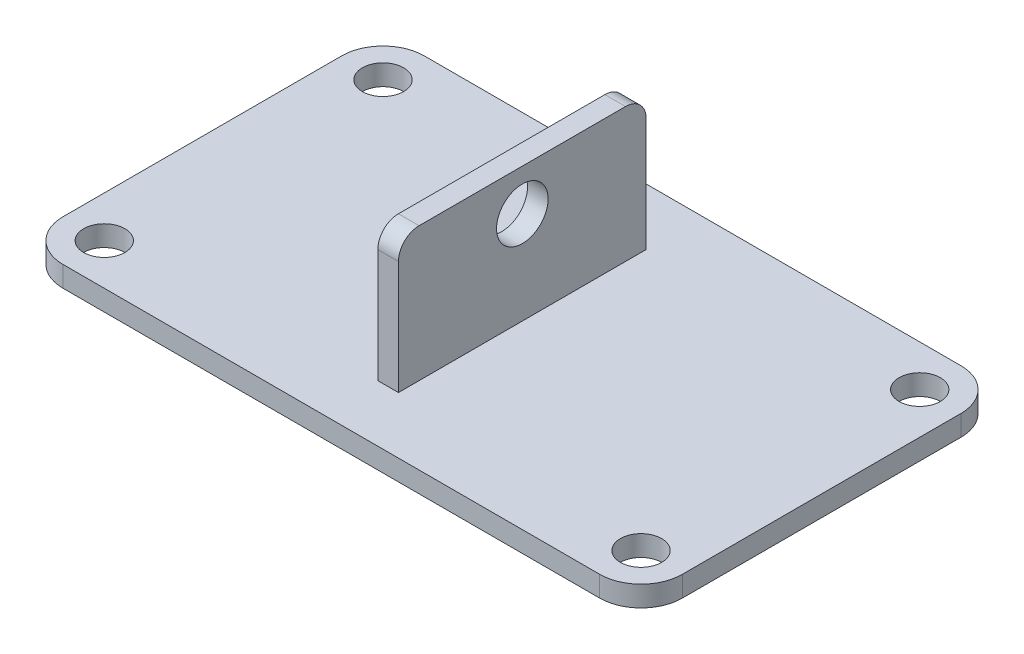
ISO-10303-21;
HEADER;
FILE_DESCRIPTION(('STEP AP214'),'2;1');
FILE_NAME('part.step','',(''),(''),'','','');
FILE_SCHEMA(('AUTOMOTIVE_DESIGN { 1 0 10303 214 1 1 1 1 }'));
ENDSEC;
DATA;
#1=APPLICATION_CONTEXT('core data for automotive mechanical design processes');
#2=APPLICATION_PROTOCOL_DEFINITION('international standard','automotive_design',2000,#1);
#3=PRODUCT_CONTEXT('',#1,'mechanical');
#4=PRODUCT('Part','Part','',(#3));
#5=PRODUCT_RELATED_PRODUCT_CATEGORY('part','',(#4));
#6=PRODUCT_DEFINITION_FORMATION('','',#4);
#7=PRODUCT_DEFINITION_CONTEXT('part definition',#1,'design');
#8=PRODUCT_DEFINITION('design','',#6,#7);
#9=PRODUCT_DEFINITION_SHAPE('','',#8);
#10=(LENGTH_UNIT() NAMED_UNIT(*) SI_UNIT(.MILLI.,.METRE.));
#11=(NAMED_UNIT(*) PLANE_ANGLE_UNIT() SI_UNIT($,.RADIAN.));
#12=(NAMED_UNIT(*) SI_UNIT($,.STERADIAN.) SOLID_ANGLE_UNIT());
#13=UNCERTAINTY_MEASURE_WITH_UNIT(LENGTH_MEASURE(1.E-05),#10,'distance_accuracy_value','');
#14=(GEOMETRIC_REPRESENTATION_CONTEXT(3) GLOBAL_UNCERTAINTY_ASSIGNED_CONTEXT((#13)) GLOBAL_UNIT_ASSIGNED_CONTEXT((#10,
#11,#12)) REPRESENTATION_CONTEXT('',''));
#15=CARTESIAN_POINT('',(0.,0.,0.));
#16=DIRECTION('',(0.,0.,1.));
#17=DIRECTION('',(1.,0.,0.));
#18=AXIS2_PLACEMENT_3D('',#15,#16,#17);
#19=CARTESIAN_POINT('',(130.,10.,-67.5));
#20=DIRECTION('',(0.,1.,0.));
#21=DIRECTION('',(0.,0.,1.));
#22=AXIS2_PLACEMENT_3D('',#19,#20,#21);
#23=PLANE('',#22);
#24=CARTESIAN_POINT('',(-130.,10.,67.5));
#25=DIRECTION('',(0.,1.,0.));
#26=DIRECTION('',(0.,0.,1.));
#27=AXIS2_PLACEMENT_3D('',#24,#25,#26);
#28=CIRCLE('',#27,9.99999999999999);
#29=CARTESIAN_POINT('',(-130.,10.,77.5));
#30=VERTEX_POINT('',#29);
#31=EDGE_CURVE('E183',#30,#30,#28,.T.);
#32=ORIENTED_EDGE('',*,*,#31,.F.);
#33=EDGE_LOOP('',(#32));
#34=FACE_BOUND('',#33,.T.);
#35=CARTESIAN_POINT('',(130.,10.,67.5));
#36=DIRECTION('',(0.,1.,0.));
#37=DIRECTION('',(0.,0.,1.));
#38=AXIS2_PLACEMENT_3D('',#35,#36,#37);
#39=CIRCLE('',#38,10.);
#40=CARTESIAN_POINT('',(130.,10.,77.5));
#41=VERTEX_POINT('',#40);
#42=EDGE_CURVE('E178',#41,#41,#39,.T.);
#43=ORIENTED_EDGE('',*,*,#42,.F.);
#44=EDGE_LOOP('',(#43));
#45=FACE_BOUND('',#44,.T.);
#46=CARTESIAN_POINT('',(130.,10.,-67.5));
#47=DIRECTION('',(0.,1.,0.));
#48=DIRECTION('',(0.,0.,1.));
#49=AXIS2_PLACEMENT_3D('',#46,#47,#48);
#50=CIRCLE('',#49,10.);
#51=CARTESIAN_POINT('',(130.,10.,-57.5));
#52=VERTEX_POINT('',#51);
#53=EDGE_CURVE('E171',#52,#52,#50,.T.);
#54=ORIENTED_EDGE('',*,*,#53,.F.);
#55=EDGE_LOOP('',(#54));
#56=FACE_BOUND('',#55,.T.);
#57=CARTESIAN_POINT('',(-130.,10.,-67.5));
#58=DIRECTION('',(0.,1.,0.));
#59=DIRECTION('',(0.,0.,1.));
#60=AXIS2_PLACEMENT_3D('',#57,#58,#59);
#61=CIRCLE('',#60,9.99999999999999);
#62=CARTESIAN_POINT('',(-130.,10.,-57.5));
#63=VERTEX_POINT('',#62);
#64=EDGE_CURVE('E172',#63,#63,#61,.T.);
#65=ORIENTED_EDGE('',*,*,#64,.F.);
#66=EDGE_LOOP('',(#65));
#67=FACE_BOUND('',#66,.T.);
#68=CARTESIAN_POINT('',(130.,10.,-67.5));
#69=DIRECTION('',(0.,1.,0.));
#70=DIRECTION('',(0.,0.,1.));
#71=AXIS2_PLACEMENT_3D('',#68,#69,#70);
#72=CIRCLE('',#71,20.);
#73=CARTESIAN_POINT('',(150.,10.,-67.4999999999999));
#74=VERTEX_POINT('',#73);
#75=CARTESIAN_POINT('',(130.,10.,-87.5));
#76=VERTEX_POINT('',#75);
#77=EDGE_CURVE('E193',#74,#76,#72,.T.);
#78=ORIENTED_EDGE('',*,*,#77,.T.);
#79=DIRECTION('',(-1.,0.,0.));
#80=VECTOR('',#79,1.);
#81=CARTESIAN_POINT('',(-130.,10.,-87.5));
#82=LINE('',#81,#80);
#83=CARTESIAN_POINT('',(-130.,10.,-87.5));
#84=VERTEX_POINT('',#83);
#85=EDGE_CURVE('E199',#76,#84,#82,.T.);
#86=ORIENTED_EDGE('',*,*,#85,.T.);
#87=CARTESIAN_POINT('',(-130.,10.,-67.5));
#88=DIRECTION('',(0.,1.,0.));
#89=DIRECTION('',(0.,0.,-1.));
#90=AXIS2_PLACEMENT_3D('',#87,#88,#89);
#91=CIRCLE('',#90,20.);
#92=CARTESIAN_POINT('',(-150.,10.,-67.4999999999999));
#93=VERTEX_POINT('',#92);
#94=EDGE_CURVE('E204',#84,#93,#91,.T.);
#95=ORIENTED_EDGE('',*,*,#94,.T.);
#96=DIRECTION('',(0.,0.,1.));
#97=VECTOR('',#96,1.);
#98=CARTESIAN_POINT('',(-150.,10.,67.4999999999998));
#99=LINE('',#98,#97);
#100=CARTESIAN_POINT('',(-150.,10.,67.4999999999998));
#101=VERTEX_POINT('',#100);
#102=EDGE_CURVE('E205',#93,#101,#99,.T.);
#103=ORIENTED_EDGE('',*,*,#102,.T.);
#104=CARTESIAN_POINT('',(-130.,10.,67.5));
#105=DIRECTION('',(0.,1.,0.));
#106=DIRECTION('',(0.,0.,-1.));
#107=AXIS2_PLACEMENT_3D('',#104,#105,#106);
#108=CIRCLE('',#107,20.);
#109=CARTESIAN_POINT('',(-130.,10.,87.5));
#110=VERTEX_POINT('',#109);
#111=EDGE_CURVE('E202',#101,#110,#108,.T.);
#112=ORIENTED_EDGE('',*,*,#111,.T.);
#113=DIRECTION('',(1.,0.,0.));
#114=VECTOR('',#113,1.);
#115=CARTESIAN_POINT('',(-130.,10.,87.5));
#116=LINE('',#115,#114);
#117=CARTESIAN_POINT('',(130.,10.,87.5));
#118=VERTEX_POINT('',#117);
#119=EDGE_CURVE('E210',#110,#118,#116,.T.);
#120=ORIENTED_EDGE('',*,*,#119,.T.);
#121=CARTESIAN_POINT('',(130.,10.,67.5));
#122=DIRECTION('',(0.,1.,0.));
#123=DIRECTION('',(0.,0.,1.));
#124=AXIS2_PLACEMENT_3D('',#121,#122,#123);
#125=CIRCLE('',#124,20.);
#126=CARTESIAN_POINT('',(150.,10.,67.4999999999998));
#127=VERTEX_POINT('',#126);
#128=EDGE_CURVE('E209',#118,#127,#125,.T.);
#129=ORIENTED_EDGE('',*,*,#128,.T.);
#130=DIRECTION('',(0.,0.,-1.));
#131=VECTOR('',#130,1.);
#132=CARTESIAN_POINT('',(150.,10.,67.4999999999998));
#133=LINE('',#132,#131);
#134=EDGE_CURVE('E212',#127,#74,#133,.T.);
#135=ORIENTED_EDGE('',*,*,#134,.T.);
#136=EDGE_LOOP('',(#78,#86,#95,#103,#112,#120,#129,#135));
#137=FACE_BOUND('',#136,.T.);
#138=DIRECTION('',(-1.,0.,0.));
#139=VECTOR('',#138,1.);
#140=CARTESIAN_POINT('',(-5.00000000000002,10.,-59.9999999999997));
#141=LINE('',#140,#139);
#142=CARTESIAN_POINT('',(4.99999999999998,10.,-59.9999999999997));
#143=VERTEX_POINT('',#142);
#144=CARTESIAN_POINT('',(-5.00000000000002,10.,-59.9999999999997));
#145=VERTEX_POINT('',#144);
#146=EDGE_CURVE('E142',#143,#145,#141,.T.);
#147=ORIENTED_EDGE('',*,*,#146,.F.);
#148=DIRECTION('',(0.,0.,-1.));
#149=VECTOR('',#148,1.);
#150=CARTESIAN_POINT('',(5.00000000000002,10.,60.0000000000003));
#151=LINE('',#150,#149);
#152=CARTESIAN_POINT('',(5.00000000000002,10.,60.0000000000003));
#153=VERTEX_POINT('',#152);
#154=EDGE_CURVE('E146',#153,#143,#151,.T.);
#155=ORIENTED_EDGE('',*,*,#154,.F.);
#156=DIRECTION('',(1.,0.,0.));
#157=VECTOR('',#156,1.);
#158=CARTESIAN_POINT('',(-5.00000000000002,10.,60.0000000000003));
#159=LINE('',#158,#157);
#160=CARTESIAN_POINT('',(-5.00000000000003,10.,60.0000000000002));
#161=VERTEX_POINT('',#160);
#162=EDGE_CURVE('E157',#161,#153,#159,.T.);
#163=ORIENTED_EDGE('',*,*,#162,.F.);
#164=DIRECTION('',(0.,0.,1.));
#165=VECTOR('',#164,1.);
#166=CARTESIAN_POINT('',(-5.00000000000002,10.,60.0000000000003));
#167=LINE('',#166,#165);
#168=EDGE_CURVE('E160',#145,#161,#167,.T.);
#169=ORIENTED_EDGE('',*,*,#168,.F.);
#170=EDGE_LOOP('',(#147,#155,#163,#169));
#171=FACE_BOUND('',#170,.T.);
#172=ADVANCED_FACE('F39',(#34,#45,#56,#67,#137,#171),#23,.T.);
#173=CARTESIAN_POINT('',(130.,10.,-67.5));
#174=DIRECTION('',(0.,-1.,0.));
#175=DIRECTION('',(0.,0.,-1.));
#176=AXIS2_PLACEMENT_3D('',#173,#174,#175);
#177=CYLINDRICAL_SURFACE('',#176,20.);
#178=CARTESIAN_POINT('',(130.,0.,-67.5));
#179=DIRECTION('',(0.,1.,0.));
#180=DIRECTION('',(0.,0.,1.));
#181=AXIS2_PLACEMENT_3D('',#178,#179,#180);
#182=CIRCLE('',#181,20.);
#183=CARTESIAN_POINT('',(150.,0.,-67.4999999999999));
#184=VERTEX_POINT('',#183);
#185=CARTESIAN_POINT('',(130.,0.,-87.5));
#186=VERTEX_POINT('',#185);
#187=EDGE_CURVE('E195',#184,#186,#182,.T.);
#188=ORIENTED_EDGE('',*,*,#187,.T.);
#189=DIRECTION('',(0.,-1.,0.));
#190=VECTOR('',#189,1.);
#191=CARTESIAN_POINT('',(130.,10.,-87.5));
#192=LINE('',#191,#190);
#193=EDGE_CURVE('E248',#76,#186,#192,.T.);
#194=ORIENTED_EDGE('',*,*,#193,.F.);
#195=ORIENTED_EDGE('',*,*,#77,.F.);
#196=DIRECTION('',(0.,-1.,0.));
#197=VECTOR('',#196,1.);
#198=CARTESIAN_POINT('',(150.,10.,-67.4999999999999));
#199=LINE('',#198,#197);
#200=EDGE_CURVE('E214',#74,#184,#199,.T.);
#201=ORIENTED_EDGE('',*,*,#200,.T.);
#202=EDGE_LOOP('',(#188,#194,#195,#201));
#203=FACE_BOUND('',#202,.T.);
#204=ADVANCED_FACE('F298',(#203),#177,.T.);
#205=CARTESIAN_POINT('',(-130.,10.,-87.5));
#206=DIRECTION('',(0.,0.,1.));
#207=DIRECTION('',(1.,0.,0.));
#208=AXIS2_PLACEMENT_3D('',#205,#206,#207);
#209=PLANE('',#208);
#210=DIRECTION('',(-1.,0.,0.));
#211=VECTOR('',#210,1.);
#212=CARTESIAN_POINT('',(-130.,0.,-87.5));
#213=LINE('',#212,#211);
#214=CARTESIAN_POINT('',(-130.,0.,-87.5));
#215=VERTEX_POINT('',#214);
#216=EDGE_CURVE('E217',#186,#215,#213,.T.);
#217=ORIENTED_EDGE('',*,*,#216,.T.);
#218=DIRECTION('',(0.,-1.,0.));
#219=VECTOR('',#218,1.);
#220=CARTESIAN_POINT('',(-130.,10.,-87.5));
#221=LINE('',#220,#219);
#222=EDGE_CURVE('E246',#84,#215,#221,.T.);
#223=ORIENTED_EDGE('',*,*,#222,.F.);
#224=ORIENTED_EDGE('',*,*,#85,.F.);
#225=ORIENTED_EDGE('',*,*,#193,.T.);
#226=EDGE_LOOP('',(#217,#223,#224,#225));
#227=FACE_BOUND('',#226,.T.);
#228=ADVANCED_FACE('F302',(#227),#209,.F.);
#229=CARTESIAN_POINT('',(-130.,10.,-67.5));
#230=DIRECTION('',(0.,-1.,0.));
#231=DIRECTION('',(0.,0.,-1.));
#232=AXIS2_PLACEMENT_3D('',#229,#230,#231);
#233=CYLINDRICAL_SURFACE('',#232,20.);
#234=CARTESIAN_POINT('',(-130.,0.,-67.5));
#235=DIRECTION('',(0.,1.,0.));
#236=DIRECTION('',(0.,0.,-1.));
#237=AXIS2_PLACEMENT_3D('',#234,#235,#236);
#238=CIRCLE('',#237,20.);
#239=CARTESIAN_POINT('',(-150.,0.,-67.4999999999999));
#240=VERTEX_POINT('',#239);
#241=EDGE_CURVE('E219',#215,#240,#238,.T.);
#242=ORIENTED_EDGE('',*,*,#241,.T.);
#243=DIRECTION('',(0.,-1.,0.));
#244=VECTOR('',#243,1.);
#245=CARTESIAN_POINT('',(-150.,10.,-67.4999999999999));
#246=LINE('',#245,#244);
#247=EDGE_CURVE('E243',#93,#240,#246,.T.);
#248=ORIENTED_EDGE('',*,*,#247,.F.);
#249=ORIENTED_EDGE('',*,*,#94,.F.);
#250=ORIENTED_EDGE('',*,*,#222,.T.);
#251=EDGE_LOOP('',(#242,#248,#249,#250));
#252=FACE_BOUND('',#251,.T.);
#253=ADVANCED_FACE('F337',(#252),#233,.T.);
#254=CARTESIAN_POINT('',(-150.,10.,67.4999999999998));
#255=DIRECTION('',(1.,0.,0.));
#256=DIRECTION('',(0.,0.,-1.));
#257=AXIS2_PLACEMENT_3D('',#254,#255,#256);
#258=PLANE('',#257);
#259=DIRECTION('',(0.,0.,1.));
#260=VECTOR('',#259,1.);
#261=CARTESIAN_POINT('',(-150.,0.,67.4999999999998));
#262=LINE('',#261,#260);
#263=CARTESIAN_POINT('',(-150.,0.,67.4999999999998));
#264=VERTEX_POINT('',#263);
#265=EDGE_CURVE('E218',#240,#264,#262,.T.);
#266=ORIENTED_EDGE('',*,*,#265,.T.);
#267=DIRECTION('',(0.,-1.,0.));
#268=VECTOR('',#267,1.);
#269=CARTESIAN_POINT('',(-150.,10.,67.4999999999998));
#270=LINE('',#269,#268);
#271=EDGE_CURVE('E239',#101,#264,#270,.T.);
#272=ORIENTED_EDGE('',*,*,#271,.F.);
#273=ORIENTED_EDGE('',*,*,#102,.F.);
#274=ORIENTED_EDGE('',*,*,#247,.T.);
#275=EDGE_LOOP('',(#266,#272,#273,#274));
#276=FACE_BOUND('',#275,.T.);
#277=ADVANCED_FACE('F331',(#276),#258,.F.);
#278=CARTESIAN_POINT('',(-130.,10.,67.5));
#279=DIRECTION('',(0.,-1.,0.));
#280=DIRECTION('',(0.,0.,-1.));
#281=AXIS2_PLACEMENT_3D('',#278,#279,#280);
#282=CYLINDRICAL_SURFACE('',#281,20.);
#283=CARTESIAN_POINT('',(-130.,0.,67.5));
#284=DIRECTION('',(0.,1.,0.));
#285=DIRECTION('',(0.,0.,-1.));
#286=AXIS2_PLACEMENT_3D('',#283,#284,#285);
#287=CIRCLE('',#286,20.);
#288=CARTESIAN_POINT('',(-130.,0.,87.5));
#289=VERTEX_POINT('',#288);
#290=EDGE_CURVE('E221',#264,#289,#287,.T.);
#291=ORIENTED_EDGE('',*,*,#290,.T.);
#292=DIRECTION('',(0.,-1.,0.));
#293=VECTOR('',#292,1.);
#294=CARTESIAN_POINT('',(-130.,10.,87.5));
#295=LINE('',#294,#293);
#296=EDGE_CURVE('E240',#110,#289,#295,.T.);
#297=ORIENTED_EDGE('',*,*,#296,.F.);
#298=ORIENTED_EDGE('',*,*,#111,.F.);
#299=ORIENTED_EDGE('',*,*,#271,.T.);
#300=EDGE_LOOP('',(#291,#297,#298,#299));
#301=FACE_BOUND('',#300,.T.);
#302=ADVANCED_FACE('F329',(#301),#282,.T.);
#303=CARTESIAN_POINT('',(-130.,10.,87.5));
#304=DIRECTION('',(0.,0.,-1.));
#305=DIRECTION('',(-1.,0.,0.));
#306=AXIS2_PLACEMENT_3D('',#303,#304,#305);
#307=PLANE('',#306);
#308=DIRECTION('',(1.,0.,0.));
#309=VECTOR('',#308,1.);
#310=CARTESIAN_POINT('',(-130.,0.,87.5));
#311=LINE('',#310,#309);
#312=CARTESIAN_POINT('',(130.,0.,87.5));
#313=VERTEX_POINT('',#312);
#314=EDGE_CURVE('E223',#289,#313,#311,.T.);
#315=ORIENTED_EDGE('',*,*,#314,.T.);
#316=DIRECTION('',(0.,-1.,0.));
#317=VECTOR('',#316,1.);
#318=CARTESIAN_POINT('',(130.,10.,87.5));
#319=LINE('',#318,#317);
#320=EDGE_CURVE('E234',#118,#313,#319,.T.);
#321=ORIENTED_EDGE('',*,*,#320,.F.);
#322=ORIENTED_EDGE('',*,*,#119,.F.);
#323=ORIENTED_EDGE('',*,*,#296,.T.);
#324=EDGE_LOOP('',(#315,#321,#322,#323));
#325=FACE_BOUND('',#324,.T.);
#326=ADVANCED_FACE('F321',(#325),#307,.F.);
#327=CARTESIAN_POINT('',(130.,10.,67.5));
#328=DIRECTION('',(0.,-1.,0.));
#329=DIRECTION('',(0.,0.,-1.));
#330=AXIS2_PLACEMENT_3D('',#327,#328,#329);
#331=CYLINDRICAL_SURFACE('',#330,20.);
#332=CARTESIAN_POINT('',(130.,0.,67.5));
#333=DIRECTION('',(0.,1.,0.));
#334=DIRECTION('',(0.,0.,1.));
#335=AXIS2_PLACEMENT_3D('',#332,#333,#334);
#336=CIRCLE('',#335,20.);
#337=CARTESIAN_POINT('',(150.,0.,67.4999999999998));
#338=VERTEX_POINT('',#337);
#339=EDGE_CURVE('E228',#313,#338,#336,.T.);
#340=ORIENTED_EDGE('',*,*,#339,.T.);
#341=DIRECTION('',(0.,-1.,0.));
#342=VECTOR('',#341,1.);
#343=CARTESIAN_POINT('',(150.,10.,67.4999999999998));
#344=LINE('',#343,#342);
#345=EDGE_CURVE('E233',#127,#338,#344,.T.);
#346=ORIENTED_EDGE('',*,*,#345,.F.);
#347=ORIENTED_EDGE('',*,*,#128,.F.);
#348=ORIENTED_EDGE('',*,*,#320,.T.);
#349=EDGE_LOOP('',(#340,#346,#347,#348));
#350=FACE_BOUND('',#349,.T.);
#351=ADVANCED_FACE('F318',(#350),#331,.T.);
#352=CARTESIAN_POINT('',(150.,10.,67.4999999999998));
#353=DIRECTION('',(-1.,0.,0.));
#354=DIRECTION('',(0.,0.,1.));
#355=AXIS2_PLACEMENT_3D('',#352,#353,#354);
#356=PLANE('',#355);
#357=DIRECTION('',(0.,0.,-1.));
#358=VECTOR('',#357,1.);
#359=CARTESIAN_POINT('',(150.,0.,67.4999999999998));
#360=LINE('',#359,#358);
#361=EDGE_CURVE('E196',#338,#184,#360,.T.);
#362=ORIENTED_EDGE('',*,*,#361,.T.);
#363=ORIENTED_EDGE('',*,*,#200,.F.);
#364=ORIENTED_EDGE('',*,*,#134,.F.);
#365=ORIENTED_EDGE('',*,*,#345,.T.);
#366=EDGE_LOOP('',(#362,#363,#364,#365));
#367=FACE_BOUND('',#366,.T.);
#368=ADVANCED_FACE('F317',(#367),#356,.F.);
#369=CARTESIAN_POINT('',(130.,0.,-67.5));
#370=DIRECTION('',(0.,1.,0.));
#371=DIRECTION('',(0.,0.,1.));
#372=AXIS2_PLACEMENT_3D('',#369,#370,#371);
#373=PLANE('',#372);
#374=CARTESIAN_POINT('',(-130.,0.,67.5));
#375=DIRECTION('',(0.,1.,0.));
#376=DIRECTION('',(0.,0.,1.));
#377=AXIS2_PLACEMENT_3D('',#374,#375,#376);
#378=CIRCLE('',#377,9.99999999999999);
#379=CARTESIAN_POINT('',(-130.,0.,77.5));
#380=VERTEX_POINT('',#379);
#381=EDGE_CURVE('E143',#380,#380,#378,.T.);
#382=ORIENTED_EDGE('',*,*,#381,.T.);
#383=EDGE_LOOP('',(#382));
#384=FACE_BOUND('',#383,.T.);
#385=CARTESIAN_POINT('',(130.,0.,67.5));
#386=DIRECTION('',(0.,1.,0.));
#387=DIRECTION('',(0.,0.,1.));
#388=AXIS2_PLACEMENT_3D('',#385,#386,#387);
#389=CIRCLE('',#388,10.);
#390=CARTESIAN_POINT('',(130.,0.,77.5));
#391=VERTEX_POINT('',#390);
#392=EDGE_CURVE('E181',#391,#391,#389,.T.);
#393=ORIENTED_EDGE('',*,*,#392,.T.);
#394=EDGE_LOOP('',(#393));
#395=FACE_BOUND('',#394,.T.);
#396=CARTESIAN_POINT('',(130.,0.,-67.5));
#397=DIRECTION('',(0.,1.,0.));
#398=DIRECTION('',(0.,0.,1.));
#399=AXIS2_PLACEMENT_3D('',#396,#397,#398);
#400=CIRCLE('',#399,10.);
#401=CARTESIAN_POINT('',(130.,0.,-57.5));
#402=VERTEX_POINT('',#401);
#403=EDGE_CURVE('E174',#402,#402,#400,.T.);
#404=ORIENTED_EDGE('',*,*,#403,.T.);
#405=EDGE_LOOP('',(#404));
#406=FACE_BOUND('',#405,.T.);
#407=CARTESIAN_POINT('',(-130.,0.,-67.5));
#408=DIRECTION('',(0.,1.,0.));
#409=DIRECTION('',(0.,0.,1.));
#410=AXIS2_PLACEMENT_3D('',#407,#408,#409);
#411=CIRCLE('',#410,9.99999999999999);
#412=CARTESIAN_POINT('',(-130.,0.,-57.5));
#413=VERTEX_POINT('',#412);
#414=EDGE_CURVE('E186',#413,#413,#411,.T.);
#415=ORIENTED_EDGE('',*,*,#414,.T.);
#416=EDGE_LOOP('',(#415));
#417=FACE_BOUND('',#416,.T.);
#418=ORIENTED_EDGE('',*,*,#187,.F.);
#419=ORIENTED_EDGE('',*,*,#361,.F.);
#420=ORIENTED_EDGE('',*,*,#339,.F.);
#421=ORIENTED_EDGE('',*,*,#314,.F.);
#422=ORIENTED_EDGE('',*,*,#290,.F.);
#423=ORIENTED_EDGE('',*,*,#265,.F.);
#424=ORIENTED_EDGE('',*,*,#241,.F.);
#425=ORIENTED_EDGE('',*,*,#216,.F.);
#426=EDGE_LOOP('',(#418,#419,#420,#421,#422,#423,#424,#425));
#427=FACE_BOUND('',#426,.T.);
#428=ADVANCED_FACE('F312',(#384,#395,#406,#417,#427),#373,.F.);
#429=CARTESIAN_POINT('',(-130.,0.,-67.5));
#430=DIRECTION('',(0.,1.,0.));
#431=DIRECTION('',(0.,0.,1.));
#432=AXIS2_PLACEMENT_3D('',#429,#430,#431);
#433=CYLINDRICAL_SURFACE('',#432,9.99999999999999);
#434=ORIENTED_EDGE('',*,*,#414,.F.);
#435=EDGE_LOOP('',(#434));
#436=FACE_BOUND('',#435,.T.);
#437=ORIENTED_EDGE('',*,*,#64,.T.);
#438=EDGE_LOOP('',(#437));
#439=FACE_BOUND('',#438,.T.);
#440=ADVANCED_FACE('F311',(#436,#439),#433,.F.);
#441=CARTESIAN_POINT('',(130.,0.,-67.5));
#442=DIRECTION('',(0.,1.,0.));
#443=DIRECTION('',(0.,0.,1.));
#444=AXIS2_PLACEMENT_3D('',#441,#442,#443);
#445=CYLINDRICAL_SURFACE('',#444,10.);
#446=ORIENTED_EDGE('',*,*,#403,.F.);
#447=EDGE_LOOP('',(#446));
#448=FACE_BOUND('',#447,.T.);
#449=ORIENTED_EDGE('',*,*,#53,.T.);
#450=EDGE_LOOP('',(#449));
#451=FACE_BOUND('',#450,.T.);
#452=ADVANCED_FACE('F365',(#448,#451),#445,.F.);
#453=CARTESIAN_POINT('',(130.,0.,67.5));
#454=DIRECTION('',(0.,1.,0.));
#455=DIRECTION('',(0.,0.,1.));
#456=AXIS2_PLACEMENT_3D('',#453,#454,#455);
#457=CYLINDRICAL_SURFACE('',#456,10.);
#458=ORIENTED_EDGE('',*,*,#392,.F.);
#459=EDGE_LOOP('',(#458));
#460=FACE_BOUND('',#459,.T.);
#461=ORIENTED_EDGE('',*,*,#42,.T.);
#462=EDGE_LOOP('',(#461));
#463=FACE_BOUND('',#462,.T.);
#464=ADVANCED_FACE('F362',(#460,#463),#457,.F.);
#465=CARTESIAN_POINT('',(-130.,0.,67.5));
#466=DIRECTION('',(0.,1.,0.));
#467=DIRECTION('',(0.,0.,1.));
#468=AXIS2_PLACEMENT_3D('',#465,#466,#467);
#469=CYLINDRICAL_SURFACE('',#468,9.99999999999999);
#470=ORIENTED_EDGE('',*,*,#381,.F.);
#471=EDGE_LOOP('',(#470));
#472=FACE_BOUND('',#471,.T.);
#473=ORIENTED_EDGE('',*,*,#31,.T.);
#474=EDGE_LOOP('',(#473));
#475=FACE_BOUND('',#474,.T.);
#476=ADVANCED_FACE('F359',(#472,#475),#469,.F.);
#477=CARTESIAN_POINT('',(5.00000000000002,75.,60.0000000000003));
#478=DIRECTION('',(-1.,0.,0.));
#479=DIRECTION('',(0.,0.,1.));
#480=AXIS2_PLACEMENT_3D('',#477,#478,#479);
#481=PLANE('',#480);
#482=CARTESIAN_POINT('',(5.,55.,0.));
#483=DIRECTION('',(1.,0.,0.));
#484=DIRECTION('',(0.,0.,-1.));
#485=AXIS2_PLACEMENT_3D('',#482,#483,#484);
#486=CIRCLE('',#485,12.5);
#487=CARTESIAN_POINT('',(4.99999999999999,55.,-12.5));
#488=VERTEX_POINT('',#487);
#489=EDGE_CURVE('E279',#488,#488,#486,.T.);
#490=ORIENTED_EDGE('',*,*,#489,.F.);
#491=EDGE_LOOP('',(#490));
#492=FACE_BOUND('',#491,.T.);
#493=DIRECTION('',(0.,-1.,0.));
#494=VECTOR('',#493,1.);
#495=CARTESIAN_POINT('',(4.99999999999998,75.,-59.9999999999997));
#496=LINE('',#495,#494);
#497=CARTESIAN_POINT('',(4.99999999999998,65.,-59.9999999999997));
#498=VERTEX_POINT('',#497);
#499=EDGE_CURVE('E136',#498,#143,#496,.T.);
#500=ORIENTED_EDGE('',*,*,#499,.F.);
#501=CARTESIAN_POINT('',(4.99999999999998,65.,-49.9999999999997));
#502=DIRECTION('',(-1.,0.,0.));
#503=DIRECTION('',(0.,0.,1.));
#504=AXIS2_PLACEMENT_3D('',#501,#502,#503);
#505=CIRCLE('',#504,10.);
#506=CARTESIAN_POINT('',(4.99999999999998,75.,-49.9999999999997));
#507=VERTEX_POINT('',#506);
#508=EDGE_CURVE('E11',#498,#507,#505,.F.);
#509=ORIENTED_EDGE('',*,*,#508,.T.);
#510=DIRECTION('',(0.,0.,-1.));
#511=VECTOR('',#510,1.);
#512=CARTESIAN_POINT('',(5.00000000000002,75.,60.0000000000003));
#513=LINE('',#512,#511);
#514=CARTESIAN_POINT('',(5.00000000000002,75.,50.0000000000003));
#515=VERTEX_POINT('',#514);
#516=EDGE_CURVE('E164',#515,#507,#513,.T.);
#517=ORIENTED_EDGE('',*,*,#516,.F.);
#518=CARTESIAN_POINT('',(5.00000000000002,65.,50.0000000000003));
#519=DIRECTION('',(-1.,0.,0.));
#520=DIRECTION('',(0.,0.,1.));
#521=AXIS2_PLACEMENT_3D('',#518,#519,#520);
#522=CIRCLE('',#521,10.);
#523=CARTESIAN_POINT('',(5.00000000000002,65.,60.0000000000003));
#524=VERTEX_POINT('',#523);
#525=EDGE_CURVE('E253',#515,#524,#522,.F.);
#526=ORIENTED_EDGE('',*,*,#525,.T.);
#527=DIRECTION('',(0.,-1.,0.));
#528=VECTOR('',#527,1.);
#529=CARTESIAN_POINT('',(5.00000000000002,75.,60.0000000000003));
#530=LINE('',#529,#528);
#531=EDGE_CURVE('E155',#524,#153,#530,.T.);
#532=ORIENTED_EDGE('',*,*,#531,.T.);
#533=ORIENTED_EDGE('',*,*,#154,.T.);
#534=EDGE_LOOP('',(#500,#509,#517,#526,#532,#533));
#535=FACE_BOUND('',#534,.T.);
#536=ADVANCED_FACE('F148',(#492,#535),#481,.F.);
#537=CARTESIAN_POINT('',(-5.00000000000002,75.,-59.9999999999997));
#538=DIRECTION('',(0.,0.,1.));
#539=DIRECTION('',(1.,0.,0.));
#540=AXIS2_PLACEMENT_3D('',#537,#538,#539);
#541=PLANE('',#540);
#542=DIRECTION('',(0.,-1.,0.));
#543=VECTOR('',#542,1.);
#544=CARTESIAN_POINT('',(-5.00000000000002,75.,-59.9999999999997));
#545=LINE('',#544,#543);
#546=CARTESIAN_POINT('',(-5.00000000000002,65.,-59.9999999999997));
#547=VERTEX_POINT('',#546);
#548=EDGE_CURVE('E147',#547,#145,#545,.T.);
#549=ORIENTED_EDGE('',*,*,#548,.F.);
#550=DIRECTION('',(-1.,0.,0.));
#551=VECTOR('',#550,1.);
#552=CARTESIAN_POINT('',(-5.00000000000002,65.,-59.9999999999997));
#553=LINE('',#552,#551);
#554=EDGE_CURVE('E48',#547,#498,#553,.F.);
#555=ORIENTED_EDGE('',*,*,#554,.T.);
#556=ORIENTED_EDGE('',*,*,#499,.T.);
#557=ORIENTED_EDGE('',*,*,#146,.T.);
#558=EDGE_LOOP('',(#549,#555,#556,#557));
#559=FACE_BOUND('',#558,.T.);
#560=ADVANCED_FACE('F138',(#559),#541,.F.);
#561=CARTESIAN_POINT('',(-5.00000000000002,75.,60.0000000000003));
#562=DIRECTION('',(1.,0.,0.));
#563=DIRECTION('',(0.,0.,-1.));
#564=AXIS2_PLACEMENT_3D('',#561,#562,#563);
#565=PLANE('',#564);
#566=CARTESIAN_POINT('',(-5.00000000000002,55.,0.));
#567=DIRECTION('',(1.,0.,0.));
#568=DIRECTION('',(0.,0.,-1.));
#569=AXIS2_PLACEMENT_3D('',#566,#567,#568);
#570=CIRCLE('',#569,12.5);
#571=CARTESIAN_POINT('',(-5.00000000000002,55.,-12.5));
#572=VERTEX_POINT('',#571);
#573=EDGE_CURVE('E43',#572,#572,#570,.T.);
#574=ORIENTED_EDGE('',*,*,#573,.T.);
#575=EDGE_LOOP('',(#574));
#576=FACE_BOUND('',#575,.T.);
#577=DIRECTION('',(0.,0.,1.));
#578=VECTOR('',#577,1.);
#579=CARTESIAN_POINT('',(-5.00000000000002,75.,60.0000000000003));
#580=LINE('',#579,#578);
#581=CARTESIAN_POINT('',(-5.00000000000002,75.,-49.9999999999997));
#582=VERTEX_POINT('',#581);
#583=CARTESIAN_POINT('',(-5.00000000000002,75.,50.0000000000003));
#584=VERTEX_POINT('',#583);
#585=EDGE_CURVE('E166',#582,#584,#580,.T.);
#586=ORIENTED_EDGE('',*,*,#585,.F.);
#587=CARTESIAN_POINT('',(-5.00000000000002,65.,-49.9999999999997));
#588=DIRECTION('',(1.,0.,0.));
#589=DIRECTION('',(0.,0.,-1.));
#590=AXIS2_PLACEMENT_3D('',#587,#588,#589);
#591=CIRCLE('',#590,10.);
#592=EDGE_CURVE('E65',#582,#547,#591,.F.);
#593=ORIENTED_EDGE('',*,*,#592,.T.);
#594=ORIENTED_EDGE('',*,*,#548,.T.);
#595=ORIENTED_EDGE('',*,*,#168,.T.);
#596=DIRECTION('',(0.,-1.,0.));
#597=VECTOR('',#596,1.);
#598=CARTESIAN_POINT('',(-5.00000000000002,75.,60.0000000000003));
#599=LINE('',#598,#597);
#600=CARTESIAN_POINT('',(-5.00000000000002,65.,60.0000000000003));
#601=VERTEX_POINT('',#600);
#602=EDGE_CURVE('E170',#601,#161,#599,.T.);
#603=ORIENTED_EDGE('',*,*,#602,.F.);
#604=CARTESIAN_POINT('',(-5.00000000000002,65.,50.0000000000003));
#605=DIRECTION('',(1.,0.,0.));
#606=DIRECTION('',(0.,0.,-1.));
#607=AXIS2_PLACEMENT_3D('',#604,#605,#606);
#608=CIRCLE('',#607,10.);
#609=EDGE_CURVE('E256',#601,#584,#608,.F.);
#610=ORIENTED_EDGE('',*,*,#609,.T.);
#611=EDGE_LOOP('',(#586,#593,#594,#595,#603,#610));
#612=FACE_BOUND('',#611,.T.);
#613=ADVANCED_FACE('F275',(#576,#612),#565,.F.);
#614=CARTESIAN_POINT('',(-5.00000000000002,75.,60.0000000000003));
#615=DIRECTION('',(0.,0.,-1.));
#616=DIRECTION('',(-1.,0.,0.));
#617=AXIS2_PLACEMENT_3D('',#614,#615,#616);
#618=PLANE('',#617);
#619=ORIENTED_EDGE('',*,*,#531,.F.);
#620=DIRECTION('',(1.,0.,0.));
#621=VECTOR('',#620,1.);
#622=CARTESIAN_POINT('',(-5.00000000000002,65.,60.0000000000003));
#623=LINE('',#622,#621);
#624=EDGE_CURVE('E260',#524,#601,#623,.F.);
#625=ORIENTED_EDGE('',*,*,#624,.T.);
#626=ORIENTED_EDGE('',*,*,#602,.T.);
#627=ORIENTED_EDGE('',*,*,#162,.T.);
#628=EDGE_LOOP('',(#619,#625,#626,#627));
#629=FACE_BOUND('',#628,.T.);
#630=ADVANCED_FACE('F346',(#629),#618,.F.);
#631=CARTESIAN_POINT('',(0.,75.,0.));
#632=DIRECTION('',(0.,-1.,0.));
#633=DIRECTION('',(0.,0.,-1.));
#634=AXIS2_PLACEMENT_3D('',#631,#632,#633);
#635=PLANE('',#634);
#636=ORIENTED_EDGE('',*,*,#516,.T.);
#637=DIRECTION('',(-1.,0.,0.));
#638=VECTOR('',#637,1.);
#639=CARTESIAN_POINT('',(0.,75.,-49.9999999999997));
#640=LINE('',#639,#638);
#641=EDGE_CURVE('E265',#507,#582,#640,.T.);
#642=ORIENTED_EDGE('',*,*,#641,.T.);
#643=ORIENTED_EDGE('',*,*,#585,.T.);
#644=DIRECTION('',(1.,0.,0.));
#645=VECTOR('',#644,1.);
#646=CARTESIAN_POINT('',(0.,75.,50.0000000000003));
#647=LINE('',#646,#645);
#648=EDGE_CURVE('E255',#584,#515,#647,.T.);
#649=ORIENTED_EDGE('',*,*,#648,.T.);
#650=EDGE_LOOP('',(#636,#642,#643,#649));
#651=FACE_BOUND('',#650,.T.);
#652=ADVANCED_FACE('F268',(#651),#635,.F.);
#653=CARTESIAN_POINT('',(0.,65.,50.0000000000003));
#654=DIRECTION('',(1.,0.,0.));
#655=DIRECTION('',(0.,0.,-1.));
#656=AXIS2_PLACEMENT_3D('',#653,#654,#655);
#657=CYLINDRICAL_SURFACE('',#656,10.);
#658=ORIENTED_EDGE('',*,*,#609,.F.);
#659=ORIENTED_EDGE('',*,*,#624,.F.);
#660=ORIENTED_EDGE('',*,*,#525,.F.);
#661=ORIENTED_EDGE('',*,*,#648,.F.);
#662=EDGE_LOOP('',(#658,#659,#660,#661));
#663=FACE_BOUND('',#662,.T.);
#664=ADVANCED_FACE('F291',(#663),#657,.T.);
#665=CARTESIAN_POINT('',(0.,65.,-49.9999999999997));
#666=DIRECTION('',(-1.,0.,0.));
#667=DIRECTION('',(0.,0.,1.));
#668=AXIS2_PLACEMENT_3D('',#665,#666,#667);
#669=CYLINDRICAL_SURFACE('',#668,10.);
#670=ORIENTED_EDGE('',*,*,#508,.F.);
#671=ORIENTED_EDGE('',*,*,#554,.F.);
#672=ORIENTED_EDGE('',*,*,#592,.F.);
#673=ORIENTED_EDGE('',*,*,#641,.F.);
#674=EDGE_LOOP('',(#670,#671,#672,#673));
#675=FACE_BOUND('',#674,.T.);
#676=ADVANCED_FACE('F41',(#675),#669,.T.);
#677=CARTESIAN_POINT('',(-60.,55.,0.));
#678=DIRECTION('',(1.,0.,0.));
#679=DIRECTION('',(0.,0.,-1.));
#680=AXIS2_PLACEMENT_3D('',#677,#678,#679);
#681=CYLINDRICAL_SURFACE('',#680,12.5);
#682=ORIENTED_EDGE('',*,*,#489,.T.);
#683=EDGE_LOOP('',(#682));
#684=FACE_BOUND('',#683,.T.);
#685=ORIENTED_EDGE('',*,*,#573,.F.);
#686=EDGE_LOOP('',(#685));
#687=FACE_BOUND('',#686,.T.);
#688=ADVANCED_FACE('F289',(#684,#687),#681,.F.);
#689=CLOSED_SHELL('',(#172,#204,#228,#253,#277,#302,#326,#351,#368,#428,#440,#452,#464,#476,
#536,#560,#613,#630,#652,#664,#676,#688));
#690=MANIFOLD_SOLID_BREP('B2',#689);
#691=ADVANCED_BREP_SHAPE_REPRESENTATION('',(#18,#690),#14);
#692=SHAPE_DEFINITION_REPRESENTATION(#9,#691);
ENDSEC;
END-ISO-10303-21;
